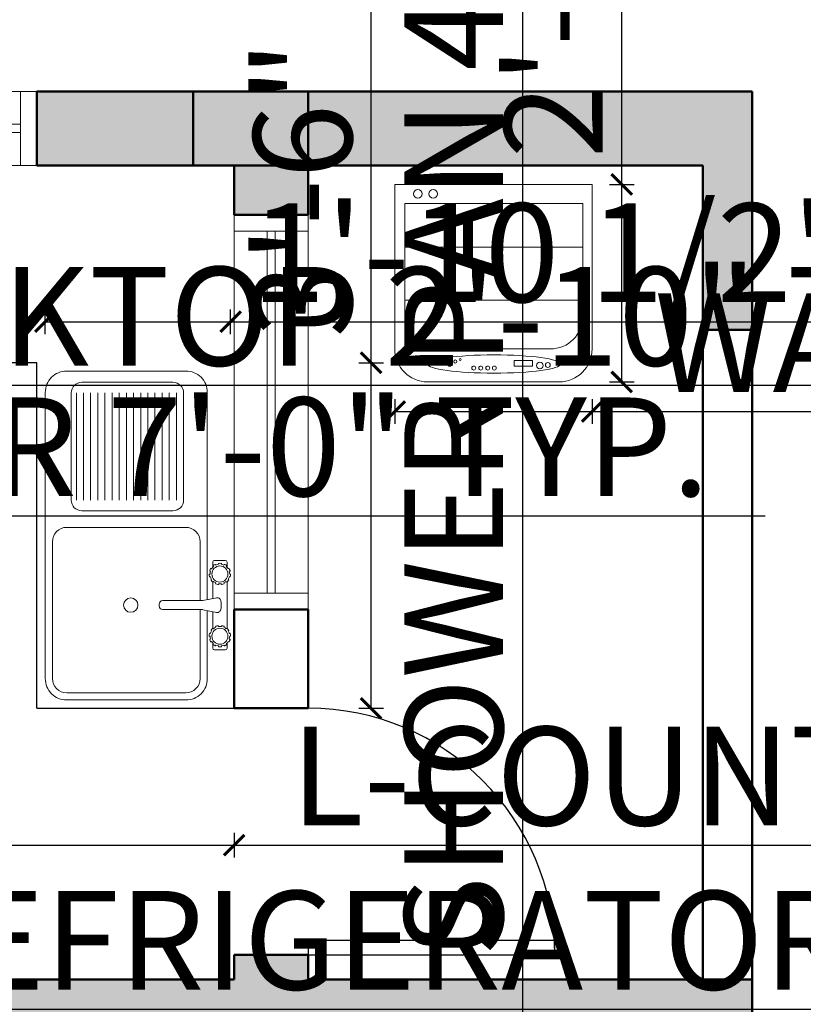
# Model space of a CAD drawing. Units: inches. Extents: x 375 to 1122, y 27 to 1069.
# Tile 153 of 155: x 897 to 992, y 872 to 991. Entities that reach past the tile are written whole.
import ezdxf

# ---------------------------------------------------------------- set-up
doc = ezdxf.new("R2010")
doc.units = ezdxf.units.IN
for name, color, linetype, lineweight in [('A-ANNO-DIMS', 2, 'Continuous', 18), ('A-COLS-PATT', 10, 'Continuous', 13), ('A-EQPM', 55, 'Continuous', 18), ('A-FLOR-FIXT', 55, 'Continuous', 18), ('A-FLOR-MILL', 55, 'Continuous', 25), ('A-WALL-PATT', 252, 'Continuous', 13), ('Columns', 10, 'Continuous', 50), ('Doors', 150, 'Continuous', 25), ('Walls', 250, 'Continuous', 50), ('Windows', 122, 'Continuous', 18)]:
    doc.layers.add(name, color=color, linetype=linetype, lineweight=lineweight)
doc.styles.get("Standard").update_dxf_attribs({"font": 'arial.ttf'})
doc.dimstyles.new('ISO-25', dxfattribs={"dimtxt": 12, "dimasz": 2.5, "dimexe": 1.5, "dimexo": 1.5, "dimtad": 1, "dimdec": 1, "dimlunit": 3, "dimtxsty": 'Standard', "dimblk": 'ARCHTICK', "dimcen": 2.5, "dimadec": 0, "dimazin": 0, "dimtfac": 1, "dimtdec": 1, "dimtmove": 0, "dimatfit": 3, "dimfxl": 1.5, "dimfxlon": 1, "dimarcsym": 0})

# ---------------------------------------------------------------- blocks, each defined once
blk = doc.blocks.new('*U13')
for p, q in [((-30, 0), (-30, -4)), ((0, 0), (0, -4))]:
    blk.add_line(p, q)
blk.add_lwpolyline([(0, 0), (0, 30), (-1.75, 30), (-1.75, 0)], close=True)
blk.add_arc((0, 0), 30, 90, 180)
blk = doc.blocks.new('TARJA2')
for p, q in [((-0.1232, -0.0169), (-0.1232, -0.0469)), ((-0.1182, -0.0119), (-0.1039, -0.0119)), ((-0.11, -0.0204), (-0.1111, -0.0199)), ((-0.1058, -0.0138), (-0.1067, -0.013)), ((-0.0999, -0.0087), (-0.1005, -0.0077)), ((-0.0928, -0.0055), (-0.0931, -0.0043)), ((-0.085, -0.0044), (-0.085, -0.0031)), ((-0.0773, -0.0055), (-0.0769, -0.0043)), ((-0.0701, -0.0087), (-0.0695, -0.0077)), ((-0.0642, -0.0138), (-0.0633, -0.013)), ((-0.0629, -0.0119), (0.0668, -0.0119)), ((-0.06, -0.0204), (-0.0589, -0.0199)), ((0.0639, -0.0204), (0.0628, -0.0199)), ((0.0682, -0.0138), (0.0672, -0.013)), ((0.0741, -0.0087), (0.0734, -0.0077)), ((0.0812, -0.0055), (0.0809, -0.0043)), ((0.0889, -0.0044), (0.0889, -0.0031)), ((0.0967, -0.0055), (0.097, -0.0043)), ((0.1038, -0.0087), (0.1045, -0.0077)), ((0.1221, -0.0119), (0.1078, -0.0119)), ((0.1097, -0.0138), (0.1107, -0.013)), ((0.114, -0.0204), (0.1151, -0.0199)), ((0.1271, -0.0169), (0.1271, -0.0469)), ((-0.1182, -0.0519), (-0.1039, -0.0519)), ((-0.1122, -0.0279), (-0.1134, -0.0278)), ((-0.1122, -0.0358), (-0.1134, -0.0359)), ((-0.11, -0.0433), (-0.1111, -0.0438)), ((-0.1058, -0.0499), (-0.1067, -0.0507)), ((-0.0999, -0.055), (-0.1005, -0.056)), ((-0.0701, -0.055), (-0.0695, -0.056)), ((-0.0642, -0.0499), (-0.0633, -0.0507)), ((-0.0629, -0.0519), (-0.0165, -0.0519)), ((-0.06, -0.0433), (-0.0589, -0.0438)), ((-0.0578, -0.0279), (-0.0566, -0.0278)), ((-0.0578, -0.0358), (-0.0566, -0.0359)), ((-0.0109, -0.0792), (-0.0187, -0.0409)), ((0.0149, -0.0792), (0.0226, -0.0409)), ((0.0204, -0.0519), (0.0668, -0.0519)), ((0.0617, -0.0279), (0.0605, -0.0278)), ((0.0617, -0.0358), (0.0605, -0.0359)), ((0.0639, -0.0433), (0.0628, -0.0438)), ((0.0682, -0.0499), (0.0672, -0.0507)), ((0.0741, -0.055), (0.0734, -0.056)), ((0.1038, -0.055), (0.1045, -0.056)), ((0.1221, -0.0519), (0.1078, -0.0519)), ((0.1097, -0.0499), (0.1107, -0.0507)), ((0.114, -0.0433), (0.1151, -0.0438)), ((0.1162, -0.0279), (0.1174, -0.0278)), ((0.1162, -0.0358), (0.1174, -0.0359)), ((-0.0928, -0.0582), (-0.0931, -0.0594)), ((-0.085, -0.0594), (-0.085, -0.0606)), ((-0.0773, -0.0582), (-0.0769, -0.0594)), ((0.0812, -0.0582), (0.0809, -0.0594)), ((0.0889, -0.0594), (0.0889, -0.0606)), ((0.0967, -0.0582), (0.097, -0.0594)), ((-0.0105, -0.0832), (-0.0105, -0.1919)), ((0.0145, -0.0832), (0.0145, -0.1919)), ((0.5952, -0.1334), (0.2956, -0.1334)), ((0.2656, -0.1634), (0.2656, -0.4178)), ((0.5952, -0.1534), (0.2956, -0.1534)), ((0.6252, -0.4178), (0.6252, -0.1634)), ((0.5952, -0.1734), (0.2956, -0.1734)), ((-0.0005, -0.2019), (0.0045, -0.2019)), ((0.5952, -0.1934), (0.2956, -0.1934)), ((0.5952, -0.2134), (0.2956, -0.2134)), ((0.5952, -0.2334), (0.2956, -0.2334)), ((0.5952, -0.2534), (0.2956, -0.2534)), ((0.5952, -0.2734), (0.2956, -0.2734)), ((0.5952, -0.2934), (0.2956, -0.2934)), ((0.5952, -0.3134), (0.2956, -0.3134)), ((0.5952, -0.3334), (0.2956, -0.3334)), ((0.5952, -0.3534), (0.2956, -0.3534)), ((0.5952, -0.3734), (0.2956, -0.3734)), ((0.5952, -0.3934), (0.2956, -0.3934)), ((0.5952, -0.4134), (0.2956, -0.4134)), ((0.5952, -0.4334), (0.2956, -0.4334)), ((0.2956, -0.4478), (0.5952, -0.4478))]:
    blk.add_line(p, q)
for points in [[(0.0173, -0.0671), (0.5964, -0.0671, -0.414214), (0.6564, -0.1271), (0.6564, -0.4602, -0.414214), (0.5964, -0.5202), (-0.2033, -0.5202, -0.414214), (-0.2633, -0.4602), (-0.2633, -0.1271, -0.414214)], [(-0.2633, -0.1271, -0.414214), (-0.2033, -0.0671), (-0.0134, -0.0671, -0.414214)], [(0.0145, -0.0871), (0.1793, -0.0871, -0.414214), (0.2193, -0.1271), (0.2193, -0.4602, -0.414214), (0.1793, -0.5002), (-0.2033, -0.5002, -0.414214), (-0.2433, -0.4602), (-0.2433, -0.1271, -0.414214)], [(-0.2433, -0.1271, -0.414214), (-0.2033, -0.0871), (-0.0105, -0.0871, -0.414214)]]:
    blk.add_lwpolyline(points, format="xyb")
for centre, radius in [((-0.085, -0.0319), 0.0225), ((0.0889, -0.0319), 0.0225), ((0.002, -0.2812), 0.02)]:
    blk.add_circle(centre, radius)
for centre, radius, start, end in [((-0.1182, -0.0169), 0.005, 90, 180), ((-0.085, -0.0319), 0.0275, 155.4545, 171.8182), ((-0.1106, -0.0188), 0.00125, 152.9626, 245.4545), ((-0.085, -0.0319), 0.03, 141.5828, 152.9626), ((-0.1075, -0.014), 0.00125, 49.0909, 141.5828), ((-0.085, -0.0319), 0.0275, 122.7273, 139.0909), ((-0.0995, -0.007), 0.00125, 120.2354, 212.7273), ((-0.085, -0.0319), 0.03, 108.8555, 120.2354), ((-0.0943, -0.0046), 0.00125, 16.3636, 108.8555), ((-0.085, -0.0319), 0.0275, 90, 106.3636), ((-0.0838, -0.0031), 0.00125, 87.5081, 180), ((-0.085, -0.0319), 0.03, 76.1283, 87.5081), ((-0.0781, -0.0039), 0.00125, 343.6364, 76.1283), ((-0.085, -0.0319), 0.0275, 57.2727, 73.6364), ((-0.0684, -0.0084), 0.00125, 54.7808, 147.2727), ((-0.085, -0.0319), 0.03, 43.401, 54.7808), ((-0.085, -0.0319), 0.0275, 24.5455, 40.9091), ((-0.0641, -0.0121), 0.00125, 310.9091, 43.401), ((-0.0584, -0.0211), 0.00125, 22.0535, 114.5455), ((-0.085, -0.0319), 0.03, 10.6737, 22.0535), ((-0.0568, -0.0265), 0.00125, 278.1818, 10.6737), ((0.0607, -0.0265), 0.00125, 169.3263, 261.8182), ((0.0889, -0.0319), 0.03, 157.9465, 169.3263), ((0.0623, -0.0211), 0.00125, 65.4545, 157.9465), ((0.0889, -0.0319), 0.0275, 139.0909, 155.4545), ((0.0681, -0.0121), 0.00125, 136.599, 229.0909), ((0.0889, -0.0319), 0.03, 125.2192, 136.599), ((0.0724, -0.0084), 0.00125, 32.7273, 125.2192), ((0.0889, -0.0319), 0.0275, 106.3636, 122.7273), ((0.0821, -0.0039), 0.00125, 103.8717, 196.3636), ((0.0889, -0.0319), 0.03, 92.4919, 103.8717), ((0.0877, -0.0031), 0.00125, 0, 92.4919), ((0.0889, -0.0319), 0.0275, 73.6364, 90), ((0.0982, -0.0046), 0.00125, 71.1445, 163.6364), ((0.0889, -0.0319), 0.03, 59.7646, 71.1445), ((0.0889, -0.0319), 0.0275, 40.9091, 57.2727), ((0.1034, -0.007), 0.00125, 327.2727, 59.7646), ((0.1115, -0.014), 0.00125, 38.4172, 130.9091), ((0.0889, -0.0319), 0.03, 27.0374, 38.4172), ((0.0889, -0.0319), 0.0275, 8.1818, 24.5455), ((0.1146, -0.0188), 0.00125, 294.5455, 27.0374), ((0.1221, -0.0169), 0.005, 0, 90), ((-0.1182, -0.0469), 0.005, 180, 270), ((-0.085, -0.0319), 0.03, 174.3101, 185.6899), ((-0.1136, -0.029), 0.00125, 81.8182, 174.3101), ((-0.1136, -0.0347), 0.00125, 185.6899, 278.1818), ((-0.085, -0.0319), 0.0275, 188.1818, 204.5455), ((-0.1106, -0.0449), 0.00125, 114.5455, 207.0374), ((-0.085, -0.0319), 0.03, 207.0374, 218.4172), ((-0.1075, -0.0497), 0.00125, 218.4172, 310.9091), ((-0.085, -0.0319), 0.0275, 220.9091, 237.2727), ((-0.085, -0.0319), 0.0275, 286.3636, 302.7273), ((-0.085, -0.0319), 0.03, 305.2192, 316.599), ((-0.085, -0.0319), 0.0275, 319.0909, 335.4545), ((-0.0641, -0.0516), 0.00125, 316.599, 49.0909), ((-0.0584, -0.0426), 0.00125, 245.4545, 337.9465), ((-0.085, -0.0319), 0.0275, 351.8182, 8.1818), ((-0.085, -0.0319), 0.03, 337.9465, 349.3263), ((-0.0568, -0.0372), 0.00125, 349.3263, 81.8182), ((-0.0089, -0.039), 0.01, 101.1605, 191.4527), ((0.002, -0.094), 0.0661, 78.8395, 101.1605), ((0.0128, -0.039), 0.01, 348.5473, 78.8395), ((0.0607, -0.0372), 0.00125, 98.1818, 190.6737), ((0.0889, -0.0319), 0.03, 190.6737, 202.0535), ((0.0623, -0.0426), 0.00125, 202.0535, 294.5455), ((0.0889, -0.0319), 0.0275, 171.8182, 188.1818), ((0.0889, -0.0319), 0.0275, 204.5455, 220.9091), ((0.0681, -0.0516), 0.00125, 130.9091, 223.401), ((0.0889, -0.0319), 0.03, 223.401, 234.7808), ((0.0889, -0.0319), 0.0275, 237.2727, 253.6364), ((0.0889, -0.0319), 0.0275, 302.7273, 319.0909), ((0.1115, -0.0497), 0.00125, 229.0909, 321.5828), ((0.0889, -0.0319), 0.03, 321.5828, 332.9626), ((0.0889, -0.0319), 0.0275, 335.4545, 351.8182), ((0.1146, -0.0449), 0.00125, 332.9626, 65.4545), ((0.1176, -0.029), 0.00125, 5.6899, 98.1818), ((0.1176, -0.0347), 0.00125, 261.8182, 354.3101), ((0.0889, -0.0319), 0.03, 354.3101, 5.6899), ((0.1221, -0.0469), 0.005, 270, 360), ((-0.0995, -0.0567), 0.00125, 147.2727, 239.7646), ((-0.085, -0.0319), 0.03, 239.7646, 251.1445), ((-0.0943, -0.0591), 0.00125, 251.1445, 343.6364), ((-0.085, -0.0319), 0.0275, 253.6364, 270), ((-0.0838, -0.0606), 0.00125, 180, 272.4919), ((-0.085, -0.0319), 0.03, 272.4919, 283.8717), ((-0.0781, -0.0598), 0.00125, 283.8717, 16.3636), ((-0.0684, -0.0553), 0.00125, 212.7273, 305.2192), ((-0.0305, -0.0832), 0.02, 0, 11.4527), ((-0.0205, -0.0822), 0.01, 0, 11.4527), ((0.0345, -0.0832), 0.02, 168.5473, 180), ((0.0724, -0.0553), 0.00125, 234.7808, 327.2727), ((0.0821, -0.0598), 0.00125, 163.6364, 256.1283), ((0.0889, -0.0319), 0.03, 256.1283, 267.5081), ((0.0877, -0.0606), 0.00125, 267.5081, 360), ((0.0889, -0.0319), 0.0275, 270, 286.3636), ((0.0982, -0.0591), 0.00125, 196.3636, 288.8555), ((0.0889, -0.0319), 0.03, 288.8555, 300.2354), ((0.1034, -0.0567), 0.00125, 300.2354, 32.7273), ((0.2956, -0.1634), 0.03, 90, 180), ((0.5952, -0.1634), 0.03, 0, 90), ((-0.0005, -0.1919), 0.01, 180, 270), ((0.0045, -0.1919), 0.01, 270, 360), ((0.2956, -0.4178), 0.03, 180, 270), ((0.5952, -0.4178), 0.03, 270, 360)]:
    blk.add_arc(centre, radius, start, end)
blk = doc.blocks.new('A$C42203764')
at = {"xscale": 1000, "yscale": 1000, "zscale": 1000}
blk.add_blockref('TARJA2', (263.3, 520.2), dxfattribs=at)
blk = doc.blocks.new('A$C20C229D7')
for p, q in [((0, 600), (0, 580)), ((24, 600), (0, 600)), ((24, 580), (24, 600)), ((22.88, 597.68), (1.21, 597.68)), ((1.21, 597.68), (1.21, 584)), ((22.88, 584), (22.88, 597.68)), ((1.21, 592.39), (22.88, 592.39)), ((1.21, 585.92), (22.88, 585.92)), ((5.21, 580), (18.88, 580)), ((14.51, 578.61), (16.76, 578.61)), ((14.51, 577.92), (14.51, 578.61)), ((16.76, 578.61), (16.76, 577.92)), ((16.76, 577.92), (14.51, 577.92)), ((4, 576), (20, 576))]:
    blk.add_line(p, q)
for centre, radius in [((2.81, 598.86), 0.52), ((4.66, 598.86), 0.52), ((6.67, 578.16), 0.267), ((7.36, 578.48), 0.187), ((7.95, 578.72), 0.133), ((17.64, 578), 0.4), ((18.62, 578.05), 0.293), ((9.61, 577.68), 0.24), ((10.46, 577.68), 0.24), ((11.31, 577.68), 0.24), ((12.11, 577.68), 0.24)]:
    blk.add_circle(centre, radius)
for centre, start, end in [((5.21, 584), 180, 270), ((18.88, 584), 270, 0), ((4, 580), 180, 270), ((20, 580), 270, 0)]:
    blk.add_arc(centre, 4, start, end)
blk.add_ellipse((12.07, 578.17), major_axis=(8.08, 0), ratio=0.137115)
blk = doc.blocks.new('_ArchTick')
at = {"color": 0, "linetype": 'ByBlock', "const_width": 0.15}
blk.add_lwpolyline([(-0.5, -0.5), (0.5, 0.5)], dxfattribs=at)
blk = doc.blocks.new('*D27')
at = {"layer": 'A-ANNO-DIMS', "color": 0, "lineweight": -2, "transparency": 16777216}
for p, q in [((444.51, 1030.21), (444.51, 1033.21)), ((986.01, 1030.21), (986.01, 1033.21)), ((444.51, 1031.71), (986.01, 1031.71))]:
    blk.add_line(p, q, dxfattribs=at)
at = {"layer": 'Defpoints', "color": 0, "transparency": 16777216}
for p in [(986.01, 1031.71), (444.51, 982.53), (986.01, 982.53)]:
    blk.add_point(p, dxfattribs=at)
at = {"layer": 'A-ANNO-DIMS', "color": 0, "lineweight": -2, "transparency": 16777216, "xscale": 2.5, "yscale": 2.5, "zscale": 2.5, "rotation": 180}
blk.add_blockref('_ArchTick', (444.51, 1031.71), dxfattribs=at)
at = {"layer": 'A-ANNO-DIMS', "color": 0, "lineweight": -2, "transparency": 16777216, "xscale": 2.5, "yscale": 2.5, "zscale": 2.5}
blk.add_blockref('_ArchTick', (986.01, 1031.71), dxfattribs=at)
at = {"layer": 'A-ANNO-DIMS', "color": 0, "transparency": 16777216, "insert": (715.26, 1038.46), "char_height": 12, "attachment_point": 5}
blk.add_mtext('45\'-1.5"', dxfattribs=at)
blk = doc.blocks.new('WINDOW-48IN')
for p, q in [((2, 5), (46, 5)), ((2, 4), (46, 4))]:
    blk.add_line(p, q)
blk.add_lwpolyline([(48, 0), (0, 0), (0, 9), (48, 9)], close=True)
for points in [[(2, 0), (2, 9)], [(46, 9), (46, 0)]]:
    blk.add_lwpolyline(points)
blk = doc.blocks.new('COLUMN-14X9IN')
blk.add_lwpolyline([(0, 0), (14, 0), (14, 9), (0, 9)], close=True)
blk = doc.blocks.new('KITCHEN-COUNTER-L')
for p, q in [((0, 9), (0, 42)), ((87, 42), (0, 42)), ((87, 0), (87, 42)), ((87, 0), (111, 0))]:
    blk.add_line(p, q)
blk = doc.blocks.new('*D61')
at = {"layer": 'A-ANNO-DIMS', "color": 0, "lineweight": -2, "transparency": 16777216}
for p, q in [((845.01, 872.43), (845.01, 869.43)), ((869.01, 872.43), (869.01, 869.43)), ((845.01, 870.93), (869.01, 870.93)), ((869.01, 870.93), (1083.13, 870.93))]:
    blk.add_line(p, q, dxfattribs=at)
at = {"layer": 'Defpoints', "color": 0, "transparency": 16777216}
for p in [(845.01, 874.53), (869.01, 874.53), (869.01, 870.93)]:
    blk.add_point(p, dxfattribs=at)
at = {"layer": 'A-ANNO-DIMS', "color": 0, "lineweight": -2, "transparency": 16777216, "xscale": 2.5, "yscale": 2.5, "zscale": 2.5, "rotation": 180}
blk.add_blockref('_ArchTick', (845.01, 870.93), dxfattribs=at)
at = {"layer": 'A-ANNO-DIMS', "color": 0, "lineweight": -2, "transparency": 16777216, "xscale": 2.5, "yscale": 2.5, "zscale": 2.5}
blk.add_blockref('_ArchTick', (869.01, 870.93), dxfattribs=at)
at = {"layer": 'A-ANNO-DIMS', "color": 0, "transparency": 16777216, "insert": (977.32, 877.76), "char_height": 12, "attachment_point": 5}
blk.add_mtext('REFRIGERATOR 2\'-0" TYP.', dxfattribs=at)
blk = doc.blocks.new('*D63')
at = {"layer": 'A-ANNO-DIMS', "color": 0, "lineweight": -2, "transparency": 16777216}
for p, q in [((894.04, 948.53), (894.04, 1069.15)), ((895.54, 948.53), (892.54, 948.53)), ((894.04, 908.53), (894.04, 948.53)), ((895.54, 908.53), (892.54, 908.53))]:
    blk.add_line(p, q, dxfattribs=at)
at = {"layer": 'Defpoints', "color": 0, "transparency": 16777216}
for p in [(894.04, 948.53), (900.04, 948.53), (900.04, 908.53)]:
    blk.add_point(p, dxfattribs=at)
at = {"layer": 'A-ANNO-DIMS', "color": 0, "lineweight": -2, "transparency": 16777216, "xscale": 2.5, "yscale": 2.5, "zscale": 2.5}
for p, rotation in [((894.04, 948.53), 90), ((894.04, 908.53), 270)]:
    blk.add_blockref('_ArchTick', p, dxfattribs=dict(at, rotation=rotation))
at = {"layer": 'A-ANNO-DIMS', "color": 0, "transparency": 16777216, "insert": (887.21, 1010.09), "char_height": 12, "attachment_point": 5, "rotation": 90}
blk.add_mtext('SINK 3\'-4" TYP.', dxfattribs=at)
blk = doc.blocks.new('*D64')
at = {"layer": 'A-ANNO-DIMS', "color": 0, "lineweight": -2, "transparency": 16777216}
for p, q in [((900.04, 953.03), (900.04, 956.03)), ((922.58, 953.03), (922.58, 956.03)), ((900.04, 954.53), (922.58, 954.53)), ((922.58, 954.53), (1035.63, 954.53))]:
    blk.add_line(p, q, dxfattribs=at)
at = {"layer": 'Defpoints', "color": 0, "transparency": 16777216}
for p in [(922.58, 954.53), (900.04, 948.53), (922.58, 948.53)]:
    blk.add_point(p, dxfattribs=at)
at = {"layer": 'A-ANNO-DIMS', "color": 0, "lineweight": -2, "transparency": 16777216, "xscale": 2.5, "yscale": 2.5, "zscale": 2.5, "rotation": 180}
blk.add_blockref('_ArchTick', (900.04, 954.53), dxfattribs=at)
at = {"layer": 'A-ANNO-DIMS', "color": 0, "lineweight": -2, "transparency": 16777216, "xscale": 2.5, "yscale": 2.5, "zscale": 2.5}
blk.add_blockref('_ArchTick', (922.58, 954.53), dxfattribs=at)
at = {"layer": 'A-ANNO-DIMS', "color": 0, "transparency": 16777216, "insert": (980.36, 961.36), "char_height": 12, "attachment_point": 5}
blk.add_mtext('1\'-10 1/2" TYP.', dxfattribs=at)
blk = doc.blocks.new('*D65')
at = {"layer": 'A-ANNO-DIMS', "color": 0, "lineweight": -2, "transparency": 16777216}
for p, q in [((942.55, 945.11), (942.55, 942.11)), ((966.55, 945.11), (966.55, 942.11)), ((942.55, 943.61), (966.55, 943.61)), ((966.55, 943.61), (1122.17, 943.61))]:
    blk.add_line(p, q, dxfattribs=at)
at = {"layer": 'Defpoints', "color": 0, "transparency": 16777216}
for p in [(942.55, 947.21), (966.55, 947.21), (966.55, 943.61)]:
    blk.add_point(p, dxfattribs=at)
at = {"layer": 'A-ANNO-DIMS', "color": 0, "lineweight": -2, "transparency": 16777216, "xscale": 2.5, "yscale": 2.5, "zscale": 2.5, "rotation": 180}
blk.add_blockref('_ArchTick', (942.55, 943.61), dxfattribs=at)
at = {"layer": 'A-ANNO-DIMS', "color": 0, "lineweight": -2, "transparency": 16777216, "xscale": 2.5, "yscale": 2.5, "zscale": 2.5}
blk.add_blockref('_ArchTick', (966.55, 943.61), dxfattribs=at)
at = {"layer": 'A-ANNO-DIMS', "color": 0, "transparency": 16777216, "insert": (1045.61, 950.44), "char_height": 12, "attachment_point": 5}
blk.add_mtext('WASHER 2\'-0" TYP.', dxfattribs=at)
blk = doc.blocks.new('*D66')
at = {"layer": 'A-ANNO-DIMS', "color": 0, "lineweight": -2, "transparency": 16777216}
for p, q in [((970.15, 971.21), (970.15, 1048.31)), ((968.65, 971.21), (971.65, 971.21)), ((970.15, 947.21), (970.15, 971.21)), ((968.65, 947.21), (971.65, 947.21))]:
    blk.add_line(p, q, dxfattribs=at)
at = {"layer": 'Defpoints', "color": 0, "transparency": 16777216}
for p in [(966.55, 971.21), (970.15, 971.21), (966.55, 947.21)]:
    blk.add_point(p, dxfattribs=at)
at = {"layer": 'A-ANNO-DIMS', "color": 0, "lineweight": -2, "transparency": 16777216, "xscale": 2.5, "yscale": 2.5, "zscale": 2.5}
for p, rotation in [((970.15, 971.21), 90), ((970.15, 947.21), 270)]:
    blk.add_blockref('_ArchTick', p, dxfattribs=dict(at, rotation=rotation))
at = {"layer": 'A-ANNO-DIMS', "color": 0, "transparency": 16777216, "insert": (963.4, 1011.01), "char_height": 12, "attachment_point": 5, "rotation": 90}
blk.add_mtext('2\'-0" TYP.', dxfattribs=at)
blk = doc.blocks.new('*D67')
at = {"layer": 'A-ANNO-DIMS', "color": 0, "lineweight": -2, "transparency": 16777216}
for p, q in [((819.23, 948.29), (819.23, 945.29)), ((853.33, 948.29), (853.33, 945.29)), ((819.23, 946.79), (853.33, 946.79)), ((853.33, 946.79), (1027.89, 946.79))]:
    blk.add_line(p, q, dxfattribs=at)
at = {"layer": 'Defpoints', "color": 0, "transparency": 16777216}
for p in [(819.23, 951.91), (853.33, 951.91), (853.33, 946.79)]:
    blk.add_point(p, dxfattribs=at)
at = {"layer": 'A-ANNO-DIMS', "color": 0, "lineweight": -2, "transparency": 16777216, "xscale": 2.5, "yscale": 2.5, "zscale": 2.5, "rotation": 180}
blk.add_blockref('_ArchTick', (819.23, 946.79), dxfattribs=at)
at = {"layer": 'A-ANNO-DIMS', "color": 0, "lineweight": -2, "transparency": 16777216, "xscale": 2.5, "yscale": 2.5, "zscale": 2.5}
blk.add_blockref('_ArchTick', (853.33, 946.79), dxfattribs=at)
at = {"layer": 'A-ANNO-DIMS', "color": 0, "transparency": 16777216, "insert": (941.86, 953.63), "char_height": 12, "attachment_point": 5}
blk.add_mtext('COOKTOP 2\'-10" TYP.', dxfattribs=at)
blk = doc.blocks.new('*D73')
at = {"layer": 'A-ANNO-DIMS', "color": 0, "lineweight": -2, "transparency": 16777216}
for p, q in [((686.76, 932.43), (686.76, 929.43)), ((770.76, 932.43), (770.76, 929.43)), ((686.76, 930.93), (770.76, 930.93)), ((770.76, 930.93), (987.61, 930.93))]:
    blk.add_line(p, q, dxfattribs=at)
at = {"layer": 'Defpoints', "color": 0, "transparency": 16777216}
for p in [(686.76, 943.53), (770.76, 943.53), (770.76, 930.93)]:
    blk.add_point(p, dxfattribs=at)
at = {"layer": 'A-ANNO-DIMS', "color": 0, "lineweight": -2, "transparency": 16777216, "xscale": 2.5, "yscale": 2.5, "zscale": 2.5, "rotation": 180}
blk.add_blockref('_ArchTick', (686.76, 930.93), dxfattribs=at)
at = {"layer": 'A-ANNO-DIMS', "color": 0, "lineweight": -2, "transparency": 16777216, "xscale": 2.5, "yscale": 2.5, "zscale": 2.5}
blk.add_blockref('_ArchTick', (770.76, 930.93), dxfattribs=at)
at = {"layer": 'A-ANNO-DIMS', "color": 0, "transparency": 16777216, "insert": (880.43, 937.76), "char_height": 12, "attachment_point": 5}
blk.add_mtext('2-PANEL SLIDER 7\'-0" TYP.', dxfattribs=at)
blk = doc.blocks.new('*D75')
at = {"layer": 'A-ANNO-DIMS', "color": 0, "lineweight": -2, "transparency": 16777216}
for p, q in [((958.11, 868.53), (958.11, 1064.59)), ((956.61, 868.53), (959.61, 868.53)), ((958.11, 814.53), (958.11, 868.53)), ((956.61, 814.53), (959.61, 814.53))]:
    blk.add_line(p, q, dxfattribs=at)
at = {"layer": 'Defpoints', "color": 0, "transparency": 16777216}
for p in [(950.01, 868.53), (958.11, 868.53), (950.01, 814.53)]:
    blk.add_point(p, dxfattribs=at)
at = {"layer": 'A-ANNO-DIMS', "color": 0, "lineweight": -2, "transparency": 16777216, "xscale": 2.5, "yscale": 2.5, "zscale": 2.5}
for p, rotation in [((958.11, 868.53), 90), ((958.11, 814.53), 270)]:
    blk.add_blockref('_ArchTick', p, dxfattribs=dict(at, rotation=rotation))
at = {"layer": 'A-ANNO-DIMS', "color": 0, "transparency": 16777216, "insert": (951.27, 967.81), "char_height": 12, "attachment_point": 5, "rotation": 90}
blk.add_mtext('SHOWER PAN 4\'-6" TYP.', dxfattribs=at)
blk = doc.blocks.new('*D77')
at = {"layer": 'A-ANNO-DIMS', "color": 0, "lineweight": -2, "transparency": 16777216}
for p, q in [((812.01, 892.38), (812.01, 889.38)), ((923.01, 892.38), (923.01, 889.38)), ((812.01, 890.88), (923.01, 890.88)), ((923.01, 890.88), (1101.82, 890.88))]:
    blk.add_line(p, q, dxfattribs=at)
at = {"layer": 'Defpoints', "color": 0, "transparency": 16777216}
for p in [(812.01, 907.53), (923.01, 907.53), (923.01, 890.88)]:
    blk.add_point(p, dxfattribs=at)
at = {"layer": 'A-ANNO-DIMS', "color": 0, "lineweight": -2, "transparency": 16777216, "xscale": 2.5, "yscale": 2.5, "zscale": 2.5, "rotation": 180}
blk.add_blockref('_ArchTick', (812.01, 890.88), dxfattribs=at)
at = {"layer": 'A-ANNO-DIMS', "color": 0, "lineweight": -2, "transparency": 16777216, "xscale": 2.5, "yscale": 2.5, "zscale": 2.5}
blk.add_blockref('_ArchTick', (923.01, 890.88), dxfattribs=at)
at = {"layer": 'A-ANNO-DIMS', "color": 0, "transparency": 16777216, "insert": (1013.66, 897.72), "char_height": 12, "attachment_point": 5}
blk.add_mtext('L-COUNTER 9\'-3" TYP.', dxfattribs=at)
blk = doc.blocks.new('*D78')
at = {"layer": 'A-ANNO-DIMS', "color": 0, "lineweight": -2, "transparency": 16777216}
for p, q in [((939.66, 949.53), (939.66, 1026.42)), ((938.16, 949.53), (941.16, 949.53)), ((939.66, 907.53), (939.66, 949.53)), ((938.16, 907.53), (941.16, 907.53))]:
    blk.add_line(p, q, dxfattribs=at)
at = {"layer": 'Defpoints', "color": 0, "transparency": 16777216}
for p in [(923.01, 949.53), (939.66, 949.53), (923.01, 907.53)]:
    blk.add_point(p, dxfattribs=at)
at = {"layer": 'A-ANNO-DIMS', "color": 0, "lineweight": -2, "transparency": 16777216, "xscale": 2.5, "yscale": 2.5, "zscale": 2.5}
for p, rotation in [((939.66, 949.53), 90), ((939.66, 907.53), 270)]:
    blk.add_blockref('_ArchTick', p, dxfattribs=dict(at, rotation=rotation))
at = {"layer": 'A-ANNO-DIMS', "color": 0, "transparency": 16777216, "insert": (932.9, 989.22), "char_height": 12, "attachment_point": 5, "rotation": 90}
blk.add_mtext('3\'-6" TYP.', dxfattribs=at)
blk = doc.blocks.new('*D83')
at = {"layer": 'A-ANNO-DIMS', "color": 0, "lineweight": -2, "transparency": 16777216}
for p, q in [((932.01, 1052.53), (932.01, 1055.53)), ((980.01, 1052.53), (980.01, 1055.53)), ((932.01, 1054.03), (980.01, 1054.03))]:
    blk.add_line(p, q, dxfattribs=at)
at = {"layer": 'Defpoints', "color": 0, "transparency": 16777216}
for p in [(980.01, 1054.03), (932.01, 973.53), (980.01, 973.53)]:
    blk.add_point(p, dxfattribs=at)
at = {"layer": 'A-ANNO-DIMS', "color": 0, "lineweight": -2, "transparency": 16777216, "xscale": 2.5, "yscale": 2.5, "zscale": 2.5, "rotation": 180}
blk.add_blockref('_ArchTick', (932.01, 1054.03), dxfattribs=at)
at = {"layer": 'A-ANNO-DIMS', "color": 0, "lineweight": -2, "transparency": 16777216, "xscale": 2.5, "yscale": 2.5, "zscale": 2.5}
blk.add_blockref('_ArchTick', (980.01, 1054.03), dxfattribs=at)
at = {"layer": 'A-ANNO-DIMS', "color": 0, "transparency": 16777216, "insert": (956.01, 1060.78), "char_height": 12, "attachment_point": 5}
blk.add_mtext('4\'-0"', dxfattribs=at)

msp = doc.modelspace()

# ---------------------------------------------------------------- hatches: boundary and pattern name
at = {"layer": 'A-COLS-PATT'}
h = msp.add_hatch(color=256, dxfattribs=at)
h.dxf.hatch_style = 1
h.paths.add_polyline_path([(512.51, 982.53), (498.51, 982.53), (498.51, 973.53), (512.51, 973.53)])
h.paths.add_polyline_path([(666.51, 982.53), (652.51, 982.53), (652.51, 973.53), (666.51, 973.53)])
h.paths.add_polyline_path([(802.01, 982.53), (788.01, 982.53), (788.01, 973.53), (802.01, 973.53)])
h.paths.add_polyline_path([(932.01, 982.53), (918.01, 982.53), (918.01, 973.53), (932.01, 973.53)])
h.paths.add_polyline_path([(507.51, 841.53), (498.51, 841.53), (498.51, 827.53), (507.51, 827.53)])
h.paths.add_polyline_path([(666.51, 844.53), (652.51, 844.53), (652.51, 835.53), (666.51, 835.53)])
h.paths.add_polyline_path([(802.01, 814.53), (788.01, 814.53), (788.01, 805.53), (802.01, 805.53)])
h.paths.add_polyline_path([(932.01, 814.53), (918.01, 814.53), (918.01, 805.53), (932.01, 805.53)])
h.paths.add_polyline_path([(507.51, 719.53), (498.51, 719.53), (498.51, 705.53), (507.51, 705.53)])
h.paths.add_polyline_path([(731.01, 676.53), (722.01, 676.53), (722.01, 662.53), (731.01, 662.53)])
h.paths.add_polyline_path([(802.01, 676.53), (788.01, 676.53), (788.01, 667.53), (802.01, 667.53)])
h.paths.add_polyline_path([(932.01, 676.53), (918.01, 676.53), (918.01, 667.53), (932.01, 667.53)])
h.paths.add_polyline_path([(932.01, 583.53), (918.01, 583.53), (918.01, 574.53), (932.01, 574.53)])
h.paths.add_polyline_path([(868.01, 583.53), (854.01, 583.53), (854.01, 574.53), (868.01, 574.53)])
h.paths.add_polyline_path([(868.01, 502.53), (854.01, 502.53), (854.01, 493.53), (868.01, 493.53)])
h.paths.add_polyline_path([(932.01, 502.53), (918.01, 502.53), (918.01, 493.53), (932.01, 493.53)])
h.paths.add_polyline_path([(672.51, 592.03), (663.51, 592.03), (663.51, 578.03), (672.51, 578.03)])
h.paths.add_polyline_path([(512.51, 589.53), (498.51, 589.53), (498.51, 580.53), (512.51, 580.53)])
h.paths.add_polyline_path([(507.51, 464.53), (498.51, 464.53), (498.51, 450.53), (507.51, 450.53)])
h.paths.add_polyline_path([(731.01, 507.53), (722.01, 507.53), (722.01, 493.53), (731.01, 493.53)])
h.paths.add_polyline_path([(802.01, 502.53), (788.01, 502.53), (788.01, 493.53), (802.01, 493.53)])
h.paths.add_polyline_path([(507.51, 342.53), (498.51, 342.53), (498.51, 328.53), (507.51, 328.53)])
h.paths.add_polyline_path([(512.51, 196.53), (498.51, 196.53), (498.51, 187.53), (512.51, 187.53)])
h.paths.add_polyline_path([(666.51, 334.53), (652.51, 334.53), (652.51, 325.53), (666.51, 325.53)])
h.paths.add_polyline_path([(666.51, 196.53), (652.51, 196.53), (652.51, 187.53), (666.51, 187.53)])
h.paths.add_polyline_path([(805.01, 196.53), (791.01, 196.53), (791.01, 187.53), (805.01, 187.53)])
h.paths.add_polyline_path([(932.01, 196.53), (918.01, 196.53), (918.01, 187.53), (932.01, 187.53)])
h.paths.add_polyline_path([(932.01, 334.53), (918.01, 334.53), (918.01, 325.53), (932.01, 325.53)])
h.paths.add_polyline_path([(805.01, 334.53), (791.01, 334.53), (791.01, 325.53), (805.01, 325.53)])
at = {"layer": 'A-WALL-PATT'}
h = msp.add_hatch(color=256, dxfattribs=at)
h.dxf.hatch_style = 1
h.paths.add_polyline_path([(962.01, 388.53), (989.01, 388.53), (989.01, 394.53), (962.01, 394.53), (932.01, 394.53), (932.01, 397.53), (923.01, 397.53), (923.01, 394.53), (842.01, 394.53), (842.01, 334.53), (839.51, 334.53), (839.51, 328.53), (854.01, 328.53), (854.01, 334.53), (848.01, 334.53), (848.01, 388.53), (953.01, 388.53), (953.01, 356.08), (962.01, 356.08), (962.01, 358.55), (989.01, 358.55), (989.01, 364.55), (962.01, 364.55)])
h.paths.add_polyline_path([(989.01, 502.53), (932.01, 502.53), (932.01, 583.53), (932.01, 593.53), (923.01, 593.53), (923.01, 583.53), (854.01, 583.53), (854.01, 556.53), (863.01, 556.53), (863.01, 574.53), (923.01, 574.53), (923.01, 502.53), (863.01, 502.53), (863.01, 520.53), (854.01, 520.53), (854.01, 502.53), (773.01, 502.53), (773.01, 493.53), (788.01, 493.53), (788.01, 402.03), (722.01, 402.03), (722.01, 373.53), (728.01, 373.53), (728.01, 396.03), (788.01, 396.03), (788.01, 373.53), (794.01, 373.53), (794.01, 430.53), (814.01, 430.53), (814.01, 436.53), (794.01, 436.53), (794.01, 493.53), (923.01, 493.53), (923.01, 487.53), (932.01, 487.53), (932.01, 493.53), (983.01, 493.53), (983.01, 473.53), (989.01, 473.53)])
h.paths.add_polyline_path([(797.01, 325.53), (805.01, 325.53), (805.01, 328.53), (807.51, 328.53), (807.51, 334.53), (791.01, 334.53), (791.01, 226.53), (770.76, 226.53), (770.76, 217.53), (791.01, 217.53), (791.01, 187.53), (855.01, 187.53), (855.01, 196.53), (797.01, 196.53)])
h.paths.add_polyline_path([(989.01, 238.53), (962.01, 238.53), (962.01, 256.42), (953.01, 256.42), (953.01, 229.53), (980.01, 229.53), (980.01, 196.53), (915.01, 196.53), (915.01, 187.53), (989.01, 187.53)])
h.paths.add_polyline_path([(962.01, 334.53), (884.01, 334.53), (884.01, 328.53), (918.01, 328.53), (918.01, 325.53), (932.01, 325.53), (932.01, 328.53), (953.01, 328.53), (953.01, 304.42), (962.01, 304.42)])
h.paths.add_polyline_path([(606.51, 283.53), (609.51, 283.53), (609.51, 289.53), (600.51, 289.53), (600.51, 196.53), (578.51, 196.53), (578.51, 187.53), (606.51, 187.53), (606.51, 196.53)])
h.paths.add_polyline_path([(666.51, 292.53), (660.51, 292.53), (660.51, 289.53), (633.51, 289.53), (633.51, 283.53), (660.51, 283.53), (660.51, 196.53), (628.01, 196.53), (628.01, 187.53), (630.53, 187.53), (630.53, 160.53), (636.53, 160.53), (636.53, 187.53), (660.51, 187.53), (660.51, 160.53), (666.51, 160.53), (666.51, 217.53), (686.76, 217.53), (686.76, 226.53), (666.51, 226.53)])
h.paths.add_polyline_path([(480.51, 256.42), (471.51, 256.42), (471.51, 238.53), (444.51, 238.53), (444.51, 187.53), (518.51, 187.53), (518.51, 196.53), (453.51, 196.53), (453.51, 229.53), (480.51, 229.53)])
h.paths.add_polyline_path([(480.51, 328.53), (652.51, 328.53), (652.51, 325.53), (660.51, 325.53), (660.51, 322.53), (666.51, 322.53), (666.51, 334.53), (507.51, 334.53), (507.51, 360.53), (498.51, 360.53), (498.51, 334.53), (471.51, 334.53), (471.51, 304.42), (480.51, 304.42)])
h.paths.add_polyline_path([(507.51, 484.53), (498.51, 484.53), (498.51, 444.53), (507.51, 444.53), (507.51, 454.53), (621.51, 454.53), (621.51, 460.53), (507.51, 460.53)])
h.paths.add_polyline_path([(672.51, 604.53), (683.26, 604.53), (683.26, 613.53), (669.51, 613.53), (669.51, 649.53), (663.51, 649.53), (663.51, 589.53), (507.51, 589.53), (507.51, 613.53), (498.51, 613.53), (498.51, 556.53), (507.51, 556.53), (507.51, 580.53), (663.51, 580.53), (663.51, 520.53), (669.51, 520.53), (669.51, 556.53), (683.26, 556.53), (683.26, 565.53), (672.51, 565.53)])
h.paths.add_polyline_path([(731.01, 667.53), (734.01, 667.53), (734.01, 676.53), (728.01, 676.53), (728.01, 715.53), (657.51, 715.53), (657.51, 709.53), (663.51, 709.53), (663.51, 673.53), (669.51, 673.53), (669.51, 709.53), (722.01, 709.53), (722.01, 613.53), (704.76, 613.53), (704.76, 604.53), (722.01, 604.53), (722.01, 565.53), (704.76, 565.53), (704.76, 556.53), (722.01, 556.53), (722.01, 502.53), (722.01, 460.53), (669.51, 460.53), (669.51, 496.53), (663.51, 496.53), (663.51, 460.53), (657.51, 460.53), (657.51, 454.53), (728.01, 454.53), (728.01, 493.53), (734.01, 493.53), (734.01, 502.53), (731.01, 502.53)])
h.paths.add_polyline_path([(986.01, 718.53), (959.01, 718.53), (959.01, 727.53), (950.01, 727.53), (950.01, 709.53), (977.01, 709.53), (977.01, 676.53), (794.01, 676.53), (794.01, 805.53), (802.01, 805.53), (802.01, 808.53), (804.51, 808.53), (804.51, 814.53), (788.01, 814.53), (788.01, 774.03), (728.01, 774.03), (728.01, 796.53), (722.01, 796.53), (722.01, 768.03), (788.01, 768.03), (788.01, 676.53), (773.01, 676.53), (773.01, 667.53), (923.01, 667.53), (923.01, 657.53), (932.01, 657.53), (932.01, 667.53), (986.01, 667.53)])
h.paths.add_polyline_path([(621.51, 715.53), (507.51, 715.53), (507.51, 733.53), (498.51, 733.53), (498.51, 715.53), (498.51, 685.53), (507.51, 685.53), (507.51, 709.53), (621.51, 709.53)])
h.paths.add_polyline_path([(666.51, 847.03), (660.51, 847.03), (660.51, 844.53), (652.51, 844.53), (652.51, 841.53), (480.51, 841.53), (480.51, 859.53), (471.51, 859.53), (471.51, 835.53), (498.51, 835.53), (498.51, 817.53), (507.51, 817.53), (507.51, 835.53), (666.51, 835.53)])
h.paths.add_polyline_path([(480.51, 940.53), (453.51, 940.53), (453.51, 973.53), (518.51, 973.53), (518.51, 982.53), (444.51, 982.53), (444.51, 931.53), (471.51, 931.53), (471.51, 907.53), (480.51, 907.53)])
h.paths.add_polyline_path([(606.51, 982.53), (578.51, 982.53), (578.51, 973.53), (600.51, 973.53), (600.51, 880.53), (609.51, 880.53), (609.51, 886.53), (606.51, 886.53)])
h.paths.add_polyline_path([(666.51, 943.53), (686.76, 943.53), (686.76, 952.53), (666.51, 952.53), (666.51, 1009.53), (660.51, 1009.53), (660.51, 982.53), (636.53, 982.53), (636.53, 1009.53), (630.53, 1009.53), (630.53, 982.53), (628.01, 982.53), (628.01, 973.53), (660.51, 973.53), (660.51, 886.53), (633.51, 886.53), (633.51, 880.53), (660.51, 880.53), (660.51, 877.03), (666.51, 877.03)])
h.paths.add_polyline_path([(986.01, 874.53), (932.01, 874.53), (932.01, 877.53), (923.01, 877.53), (923.01, 874.53), (788.01, 874.53), (788.01, 868.53), (788.01, 844.53), (794.01, 844.53), (794.01, 868.53), (839.01, 868.53), (839.01, 814.53), (836.51, 814.53), (836.51, 808.53), (851.01, 808.53), (851.01, 814.53), (845.01, 814.53), (845.01, 868.53), (986.01, 868.53)])
h.paths.add_polyline_path([(959.01, 838.55), (986.01, 838.55), (986.01, 844.55), (959.01, 844.55), (959.01, 847.03), (950.01, 847.03), (950.01, 814.53), (881.01, 814.53), (881.01, 808.53), (918.01, 808.53), (918.01, 805.53), (932.01, 805.53), (932.01, 808.53), (950.01, 808.53), (950.01, 793.53), (959.01, 793.53)])
h.paths.add_polyline_path([(986.01, 982.53), (899.01, 982.53), (899.01, 973.53), (923.01, 973.53), (923.01, 967.53), (932.01, 967.53), (932.01, 973.53), (980.01, 973.53), (980.01, 953.53), (986.01, 953.53)])
h.paths.add_polyline_path([(851.01, 982.53), (788.01, 982.53), (788.01, 952.53), (770.76, 952.53), (770.76, 943.53), (788.01, 943.53), (788.01, 910.53), (814.01, 910.53), (814.01, 916.53), (794.01, 916.53), (794.01, 973.53), (851.01, 973.53)])

# ---------------------------------------------------------------- linework, layer by layer
at = {"layer": 'Walls'}
for p, q in [((986.01, 982.53), (899.01, 982.53)), ((899.01, 973.53), (899.01, 982.53)), ((986.01, 874.53), (986.01, 982.53)), ((923.01, 973.53), (899.01, 973.53)), ((923.01, 967.53), (923.01, 973.53)), ((980.01, 973.53), (932.01, 973.53)), ((932.01, 967.53), (932.01, 973.53)), ((980.01, 874.53), (980.01, 973.53)), ((932.01, 967.53), (923.01, 967.53)), ((980.01, 953.53), (986.01, 953.53)), ((923.01, 907.53), (923.01, 919.53)), ((932.01, 919.53), (923.01, 919.53)), ((932.01, 907.53), (932.01, 919.53)), ((932.01, 907.53), (923.01, 907.53)), ((923.01, 874.53), (923.01, 877.53)), ((932.01, 877.53), (923.01, 877.53)), ((932.01, 874.53), (932.01, 877.53)), ((923.01, 874.53), (788.01, 874.53)), ((986.01, 874.53), (932.01, 874.53)), ((986.01, 874.53), (986.01, 868.53))]:
    msp.add_line(p, q, dxfattribs=at)

# ---------------------------------------------------------------- block references
at = {"layer": 'A-EQPM'}
msp.add_blockref('A$C20C229D7', (942.55, 371.21), dxfattribs=at)
at = {"layer": 'A-FLOR-FIXT', "xscale": -0.0434894164314068, "yscale": 0.0434894164314068, "zscale": 0.0434894164314068, "rotation": 270}
msp.add_blockref('A$C42203764', (900.04, 908.53), dxfattribs=at)
at = {"layer": 'A-FLOR-MILL'}
msp.add_blockref('KITCHEN-COUNTER-L', (812.01, 907.53), dxfattribs=at)
at = {"layer": 'Columns'}
msp.add_blockref('COLUMN-14X9IN', (918.01, 973.53), dxfattribs=at)
at = {"layer": 'Doors', "rotation": 270}
msp.add_blockref('*U13', (932.01, 877.53), dxfattribs=at)
at = {"layer": 'Windows'}
msp.add_blockref('WINDOW-48IN', (851.01, 973.53), dxfattribs=at)
at = {"layer": 'Windows', "rotation": 90}
msp.add_blockref('WINDOW-48IN', (932.01, 919.53), dxfattribs=at)

# ---------------------------------------------------------------- dimensions: what is measured, and where the dimension line sits
at = {"layer": 'A-ANNO-DIMS'}
for base, p1, p2, text, picture, middle in [((894.04, 948.53), (900.04, 908.53), (900.04, 948.53), 'SINK <> TYP.', '*D63', (887.21, 1010.09)), ((958.11, 868.53), (950.01, 814.53), (950.01, 868.53), 'SHOWER PAN <> TYP.', '*D75', (951.27, 967.81)), ((970.15, 971.21), (966.55, 947.21), (966.55, 971.21), '<> TYP.', '*D66', (963.4, 1011.01)), ((939.66, 949.53), (923.01, 907.53), (923.01, 949.53), '<> TYP.', '*D78', (932.9, 989.22))]:
    dim = msp.add_linear_dim(base=base, p1=p1, p2=p2, angle=90, text=text, dimstyle='ISO-25', override={"dimdec": 1, "dimlfac": 1, "dimrnd": 0, "dimzin": 1, "dimdsep": 46, "dimlunit": 4, "dimfrac": 2}, dxfattribs=at)
    dim.commit()
    dim.dimension.update_dxf_attribs({"geometry": picture, "text_midpoint": middle})
dim = msp.add_linear_dim(base=(980.01, 1054.03), p1=(932.01, 973.53), p2=(980.01, 973.53), dimstyle='ISO-25', override={"dimdec": 1, "dimlfac": 1, "dimrnd": 0, "dimzin": 1, "dimdsep": 46, "dimlunit": 4, "dimfrac": 2}, dxfattribs=at)
dim.commit()
dim.dimension.update_dxf_attribs({"geometry": '*D83', "text_midpoint": (956.01, 1060.78)})
dim = msp.add_linear_dim(base=(986.01, 1031.71), p1=(444.51, 982.53), p2=(986.01, 982.53), dimstyle='ISO-25', override={"dimclrd": 0, "dimclre": 0, "dimclrt": 0}, dxfattribs=at)
dim.commit()
dim.dimension.update_dxf_attribs({"geometry": '*D27', "text_midpoint": (715.26, 1031.71), "dimtype": 160})
for base, p1, p2, text, picture, middle in [((922.58, 954.53), (900.04, 948.53), (922.58, 948.53), '<> TYP.', '*D64', (980.36, 961.36)), ((853.33, 946.79), (819.23, 951.91), (853.33, 951.91), 'COOKTOP <> TYP.', '*D67', (941.86, 953.63)), ((966.55, 943.61), (942.55, 947.21), (966.55, 947.21), 'WASHER <> TYP.', '*D65', (1045.61, 950.44)), ((770.76, 930.93), (686.76, 943.53), (770.76, 943.53), '2-PANEL SLIDER <> TYP.', '*D73', (880.43, 937.76)), ((923.01, 890.88), (812.01, 907.53), (923.01, 907.53), 'L-COUNTER <> TYP.', '*D77', (1013.66, 897.72)), ((869.01, 870.93), (845.01, 874.53), (869.01, 874.53), 'REFRIGERATOR <> TYP.', '*D61', (977.32, 877.76))]:
    dim = msp.add_linear_dim(base=base, p1=p1, p2=p2, text=text, dimstyle='ISO-25', override={"dimdec": 1, "dimlfac": 1, "dimrnd": 0, "dimzin": 1, "dimdsep": 46, "dimlunit": 4, "dimfrac": 2}, dxfattribs=at)
    dim.commit()
    dim.dimension.update_dxf_attribs({"geometry": picture, "text_midpoint": middle})

doc.saveas('drawing.dxf')
